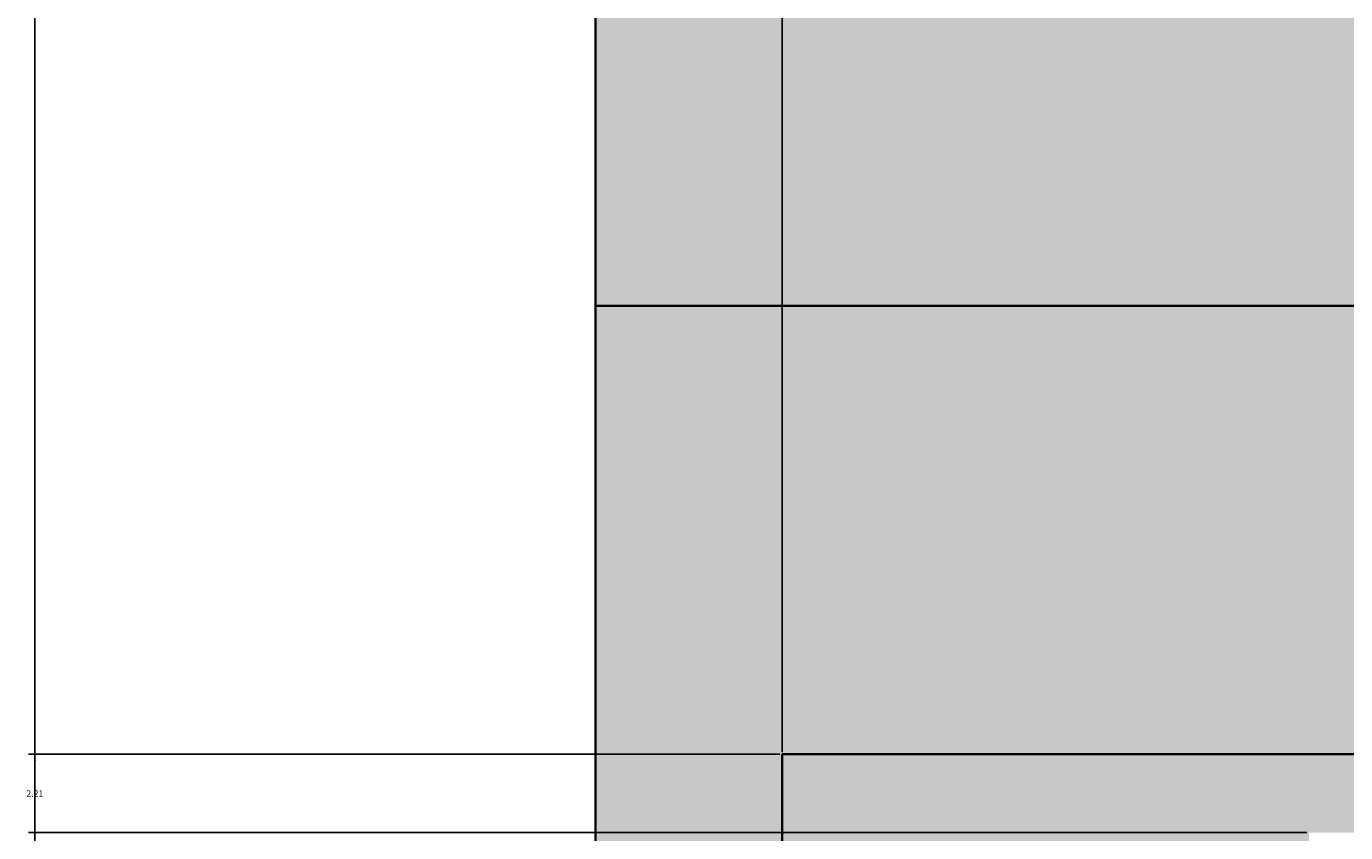
# Model space of a CAD drawing. Units: feet. Extents: x 2695 to 2912, y 795 to 1139.
# Tile 45 of 83: x 2695 to 2732, y 1048 to 1071. Entities that reach past the tile are written whole.
import ezdxf

# ---------------------------------------------------------------- set-up
doc = ezdxf.new("R2010")
doc.units = ezdxf.units.FT
for name, color, linetype, lineweight in [('A-ANNO-DIMS', 2, 'Continuous', 18), ('A-ELEV', 7, 'Continuous', 35), ('A-ELEV-PATT', 252, 'Continuous', 13)]:
    doc.layers.add(name, color=color, linetype=linetype, lineweight=lineweight)
doc.styles.get("Standard").update_dxf_attribs({"font": 'arial.ttf'})
doc.dimstyles.get("Standard").update_dxf_attribs({"dimtxt": 0.18, "dimasz": 0.18, "dimexe": 0.18, "dimexo": 0.0625, "dimgap": 0.09, "dimtad": 0, "dimtih": 1, "dimtoh": 1, "dimdec": 1, "dimzin": 0, "dimdsep": 46, "dimlunit": 3, "dimtxsty": 'Standard', "dimcen": 0.09, "dimadec": 0, "dimazin": 0, "dimtfac": 1, "dimtdec": 1, "dimtofl": 0, "dimtmove": 0, "dimatfit": 3, "dimfxl": 1, "dimtolj": 1, "dimtzin": 0, "dimarcsym": 0})

# ---------------------------------------------------------------- blocks, each defined once
blk = doc.blocks.new('*D7')
at = {"layer": 'A-ANNO-DIMS', "color": 0, "lineweight": -2, "transparency": 16777216}
for p, q in [((2710.636, 1122.993), (2710.636, 1138.886)), ((2715.885, 1050.373), (2715.885, 1138.886)), ((2710.816, 1138.706), (2712.867, 1138.706)), ((2715.705, 1138.706), (2713.655, 1138.706))]:
    blk.add_line(p, q, dxfattribs=at)
at = {"layer": 'A-ANNO-DIMS', "color": 0, "transparency": 16777216}
for points in [[(2710.816, 1138.736), (2710.816, 1138.676), (2710.636, 1138.706)], [(2715.705, 1138.736), (2715.705, 1138.676), (2715.885, 1138.706)]]:
    blk.add_solid(points, dxfattribs=at)
at = {"layer": 'Defpoints', "color": 0, "transparency": 16777216}
for p in [(2715.885, 1138.706), (2710.636, 1122.931), (2715.885, 1050.311)]:
    blk.add_point(p, dxfattribs=at)
at = {"layer": 'A-ANNO-DIMS', "color": 0, "transparency": 16777216, "insert": (2713.261, 1138.706), "char_height": 0.18, "attachment_point": 5}
blk.add_mtext('\\A1;5.249', dxfattribs=at)
blk = doc.blocks.new('*D8')
at = {"layer": 'A-ANNO-DIMS', "color": 0, "lineweight": -2, "transparency": 16777216}
for p, q in [((2715.885, 1050.373), (2715.885, 1138.886)), ((2770.636, 1122.993), (2770.636, 1138.886)), ((2716.065, 1138.706), (2742.866, 1138.706)), ((2770.456, 1138.706), (2743.655, 1138.706))]:
    blk.add_line(p, q, dxfattribs=at)
at = {"layer": 'A-ANNO-DIMS', "color": 0, "transparency": 16777216}
for points in [[(2716.065, 1138.736), (2716.065, 1138.676), (2715.885, 1138.706)], [(2770.456, 1138.736), (2770.456, 1138.676), (2770.636, 1138.706)]]:
    blk.add_solid(points, dxfattribs=at)
at = {"layer": 'Defpoints', "color": 0, "transparency": 16777216}
for p in [(2770.636, 1138.706), (2770.636, 1122.931), (2715.885, 1050.311)]:
    blk.add_point(p, dxfattribs=at)
at = {"layer": 'A-ANNO-DIMS', "color": 0, "transparency": 16777216, "insert": (2743.261, 1138.706), "char_height": 0.18, "attachment_point": 5}
blk.add_mtext('\\A1;54.75', dxfattribs=at)
blk = doc.blocks.new('*D12')
at = {"layer": 'A-ANNO-DIMS', "color": 0, "lineweight": -2, "transparency": 16777216}
for p, q in [((2710.574, 1122.931), (2694.681, 1122.931)), ((2694.861, 1122.751), (2694.861, 967.113)), ((2694.861, 811.111), (2694.861, 966.749)), ((2710.574, 810.931), (2694.681, 810.931))]:
    blk.add_line(p, q, dxfattribs=at)
at = {"layer": 'A-ANNO-DIMS', "color": 0, "transparency": 16777216}
for points in [[(2694.831, 1122.751), (2694.891, 1122.751), (2694.861, 1122.931)], [(2694.831, 811.111), (2694.891, 811.111), (2694.861, 810.931)]]:
    blk.add_solid(points, dxfattribs=at)
at = {"layer": 'Defpoints', "color": 0, "transparency": 16777216}
for p in [(2694.861, 1122.931), (2710.636, 1122.931), (2710.636, 810.931)]:
    blk.add_point(p, dxfattribs=at)
at = {"layer": 'A-ANNO-DIMS', "color": 0, "transparency": 16777216, "insert": (2694.861, 966.931), "char_height": 0.18, "attachment_point": 5}
blk.add_mtext('\\A1;312', dxfattribs=at)
blk = doc.blocks.new('*D46')
at = {"layer": 'A-ANNO-DIMS', "color": 0, "lineweight": -2, "transparency": 16777216}
for p, q in [((2730.646, 1048.105), (2694.681, 1048.105)), ((2694.861, 1047.925), (2694.861, 1047.493)), ((2694.861, 1046.698), (2694.861, 1047.13)), ((2730.646, 1046.518), (2694.681, 1046.518))]:
    blk.add_line(p, q, dxfattribs=at)
at = {"layer": 'A-ANNO-DIMS', "color": 0, "transparency": 16777216}
for points in [[(2694.831, 1047.925), (2694.891, 1047.925), (2694.861, 1048.105)], [(2694.831, 1046.698), (2694.891, 1046.698), (2694.861, 1046.518)]]:
    blk.add_solid(points, dxfattribs=at)
at = {"layer": 'Defpoints', "color": 0, "transparency": 16777216}
for p in [(2694.861, 1048.105), (2730.708, 1048.105), (2730.708, 1046.518)]:
    blk.add_point(p, dxfattribs=at)
at = {"layer": 'A-ANNO-DIMS', "color": 0, "transparency": 16777216, "insert": (2694.861, 1047.312), "char_height": 0.18, "attachment_point": 5}
blk.add_mtext('\\A1;1.59', dxfattribs=at)
blk = doc.blocks.new('*D47')
at = {"layer": 'A-ANNO-DIMS', "color": 0, "lineweight": -2, "transparency": 16777216}
for p, q in [((2715.823, 1050.311), (2694.681, 1050.311)), ((2694.861, 1050.131), (2694.861, 1049.388)), ((2694.861, 1048.285), (2694.861, 1049.027)), ((2730.646, 1048.105), (2694.681, 1048.105))]:
    blk.add_line(p, q, dxfattribs=at)
at = {"layer": 'A-ANNO-DIMS', "color": 0, "transparency": 16777216}
for points in [[(2694.831, 1050.131), (2694.891, 1050.131), (2694.861, 1050.311)], [(2694.831, 1048.285), (2694.891, 1048.285), (2694.861, 1048.105)]]:
    blk.add_solid(points, dxfattribs=at)
at = {"layer": 'Defpoints', "color": 0, "transparency": 16777216}
for p in [(2694.861, 1050.311), (2715.885, 1050.311), (2730.708, 1048.105)]:
    blk.add_point(p, dxfattribs=at)
at = {"layer": 'A-ANNO-DIMS', "color": 0, "transparency": 16777216, "insert": (2694.861, 1049.208), "char_height": 0.18, "attachment_point": 5}
blk.add_mtext('\\A1;2.21', dxfattribs=at)

msp = doc.modelspace()

# ---------------------------------------------------------------- hatches: boundary and pattern name
at = {"layer": 'A-ELEV-PATT'}
h = msp.add_hatch(color=256, dxfattribs=at)
h.set_gradient(color1=(255, 255, 255), tint=1)
h.paths.add_polyline_path([(2770.6361, 1122.9306), (2710.6361, 1122.9306), (2710.6361, 1118.4096), (2770.6361, 1118.4096)])
h.paths.add_polyline_path([(2890.6361, 1107.8588), (2770.6361, 1107.8588), (2770.6361, 1103.3378), (2890.6361, 1103.3378)])
h.paths.add_polyline_path([(2890.6361, 1062.9306), (2710.6361, 1062.9306), (2710.6361, 1056.9306), (2710.6361, 936.9306), (2710.6361, 924.3105), (2716.5358, 924.3105), (2890.6361, 924.3105), (2890.6361, 936.9306), (2715.8852, 936.9306), (2715.8852, 1050.3105), (2890.6361, 1050.3105)])
h.paths.add_polyline_path([(2716.5358, 924.3105), (2710.6361, 924.3105), (2710.6361, 810.9306), (2716.5358, 810.9306)])
h = msp.add_hatch(color=256, dxfattribs=at)
h.set_gradient(color1=(147, 149, 152), color2=(147, 149, 152), tint=1)
h.paths.add_polyline_path([(2770.6361, 1118.4096), (2710.6361, 1118.4096), (2710.6361, 1062.9306), (2770.6361, 1062.9306)])
h.paths.add_polyline_path([(2890.6361, 1103.3378), (2770.6361, 1103.3378), (2770.6361, 1062.9306), (2890.6361, 1062.9306)])
h.paths.add_polyline_path([(2730.7081, 1048.1052), (2755.1125, 1048.1052), (2755.1125, 936.9306), (2770.6361, 936.9306), (2770.6361, 1050.3105), (2715.8852, 1050.3105), (2715.8852, 936.9306), (2730.7081, 936.9306)])
h.paths.add_polyline_path([(2890.6361, 1050.3105), (2770.6361, 1050.3105), (2770.6361, 971.9673), (2778.0341, 971.9673), (2778.0341, 1020.8235), (2843.575, 1020.8235), (2843.575, 971.9673), (2890.6361, 971.9673)])
h.paths.add_polyline_path([(2888.1882, 970.7156), (2843.575, 970.7156), (2843.575, 964.8267), (2888.1882, 964.8267)])
h.paths.add_polyline_path([(2888.1882, 964.1328), (2843.575, 964.1328), (2843.575, 956.614), (2888.1882, 956.614)])
h.paths.add_polyline_path([(2888.1882, 955.9202), (2843.575, 955.9202), (2843.575, 949.2892), (2888.1882, 949.2892)])
h.paths.add_polyline_path([(2888.1882, 948.5954), (2843.575, 948.5954), (2843.575, 941.3507), (2888.1882, 941.3507)])
h.paths.add_polyline_path([(2888.1882, 940.6569), (2843.575, 940.6569), (2843.575, 936.9306), (2888.1882, 936.9306)])
h.paths.add_polyline_path([(2890.6361, 970.7156), (2888.9368, 970.7156), (2888.9368, 964.8267), (2890.6361, 964.8267)])
h.paths.add_polyline_path([(2890.6361, 964.1328), (2888.9368, 964.1328), (2888.9368, 956.614), (2890.6361, 956.614)])
h.paths.add_polyline_path([(2890.6361, 955.9202), (2888.9368, 955.9202), (2888.9368, 949.2892), (2890.6361, 949.2892)])
h.paths.add_polyline_path([(2890.6361, 940.6569), (2888.9368, 940.6569), (2888.9368, 936.9306), (2890.6361, 936.9306)])
h.paths.add_polyline_path([(2890.6361, 948.5954), (2888.9368, 948.5954), (2888.9368, 941.3507), (2890.6361, 941.3507)])
h.paths.add_polyline_path([(2772.5216, 970.7156), (2770.6361, 970.7156), (2770.6361, 964.8267), (2772.5216, 964.8267)])
h.paths.add_polyline_path([(2772.5216, 964.1328), (2770.6361, 964.1328), (2770.6361, 956.614), (2772.5216, 956.614)])
h.paths.add_polyline_path([(2772.5216, 955.9202), (2770.6361, 955.9202), (2770.6361, 949.2892), (2772.5216, 949.2892)])
h.paths.add_polyline_path([(2772.5216, 948.5954), (2770.6361, 948.5954), (2770.6361, 941.3507), (2772.5216, 941.3507)])
h.paths.add_polyline_path([(2772.5216, 940.6569), (2770.6361, 940.6569), (2770.6361, 936.9306), (2772.5216, 936.9306)])
h.paths.add_polyline_path([(2778.0341, 940.6569), (2773.2702, 940.6569), (2773.2702, 936.9306), (2778.0341, 936.9306)])
h.paths.add_polyline_path([(2778.0341, 970.7156), (2773.2702, 970.7156), (2773.2702, 964.8267), (2778.0341, 964.8267)])
h.paths.add_polyline_path([(2778.0341, 964.1328), (2773.2702, 964.1328), (2773.2702, 956.614), (2778.0341, 956.614)])
h.paths.add_polyline_path([(2778.0341, 955.9202), (2773.2702, 955.9202), (2773.2702, 949.2892), (2778.0341, 949.2892)])
h.paths.add_polyline_path([(2778.0341, 948.5954), (2773.2702, 948.5954), (2773.2702, 941.3507), (2778.0341, 941.3507)])
h.paths.add_polyline_path([(2810.0407, 940.6569), (2780.0341, 940.6569), (2780.0341, 936.9306), (2810.0407, 936.9306)])
h.paths.add_polyline_path([(2890.6361, 924.3105), (2770.6361, 924.3105), (2770.6361, 810.9306), (2773.5029, 810.9306), (2773.5029, 905.5143), (2805.9398, 905.5143), (2838.3767, 905.5143), (2838.3767, 810.9306), (2890.6361, 810.9306)])

# ---------------------------------------------------------------- linework, layer by layer
at = {"layer": 'A-ELEV'}
for p, q in [((2710.6361, 1062.9306), (2710.6361, 1122.9306)), ((2710.6361, 1118.4096), (2710.6361, 1062.9306)), ((2710.6361, 1056.9306), (2710.6361, 1062.9306)), ((2710.6361, 1062.9306), (2890.6361, 1062.9306)), ((2710.6361, 1062.9306), (2895.4694, 1062.9306)), ((2710.6361, 936.9306), (2710.6361, 1056.9306)), ((2890.6361, 1050.3105), (2715.8852, 1050.3105)), ((2715.8852, 1050.3105), (2715.8852, 936.9306))]:
    msp.add_line(p, q, dxfattribs=at)
for points in [[(2715.8852, 1050.3105), (2715.8852, 936.9306)], [(2890.6361, 1050.3105), (2715.8852, 1050.3105)]]:
    msp.add_lwpolyline(points, dxfattribs=at)

# ---------------------------------------------------------------- dimensions: what is measured, and where the dimension line sits
at = {"layer": 'A-ANNO-DIMS'}
for base, p1, p2, override, picture, middle in [((2715.8852, 1138.7056), (2710.6361, 1122.9306), (2715.8852, 1050.3105), {"dimdec": 3, "dimlfac": 1, "dimrnd": 0, "dimzin": 0, "dimdsep": 46, "dimlunit": 2}, '*D7', (2713.2606, 1138.7056)), ((2770.6361, 1138.7056), (2715.8852, 1050.3105), (2770.6361, 1122.9306), {"dimdec": 2, "dimlfac": 1, "dimrnd": 0, "dimzin": 0, "dimdsep": 46, "dimlunit": 2}, '*D8', (2743.2606, 1138.7056))]:
    dim = msp.add_linear_dim(base=base, p1=p1, p2=p2, dimstyle='Standard', override=override, dxfattribs=at)
    dim.commit()
    dim.dimension.update_dxf_attribs({"geometry": picture, "text_midpoint": middle})
for base, p1, p2, override, picture, middle in [((2694.8611, 1122.9306), (2710.6361, 810.9306), (2710.6361, 1122.9306), {"dimdec": 0, "dimlfac": 1, "dimrnd": 0, "dimzin": 0, "dimdsep": 46, "dimlunit": 2}, '*D12', (2694.8611, 966.9306)), ((2694.8611, 1050.3105), (2730.7081, 1048.1052), (2715.8852, 1050.3105), {"dimdec": 2, "dimlfac": 1, "dimrnd": 0, "dimzin": 0, "dimdsep": 46, "dimlunit": 2}, '*D47', (2694.8611, 1049.2079)), ((2694.8611, 1048.1052), (2730.7081, 1046.5179), (2730.7081, 1048.1052), {"dimdec": 2, "dimlfac": 1, "dimrnd": 0, "dimzin": 0, "dimdsep": 46, "dimlunit": 2}, '*D46', (2694.8611, 1047.3116))]:
    dim = msp.add_linear_dim(base=base, p1=p1, p2=p2, angle=90, dimstyle='Standard', override=override, dxfattribs=at)
    dim.commit()
    dim.dimension.update_dxf_attribs({"geometry": picture, "text_midpoint": middle})

doc.saveas('drawing.dxf')
